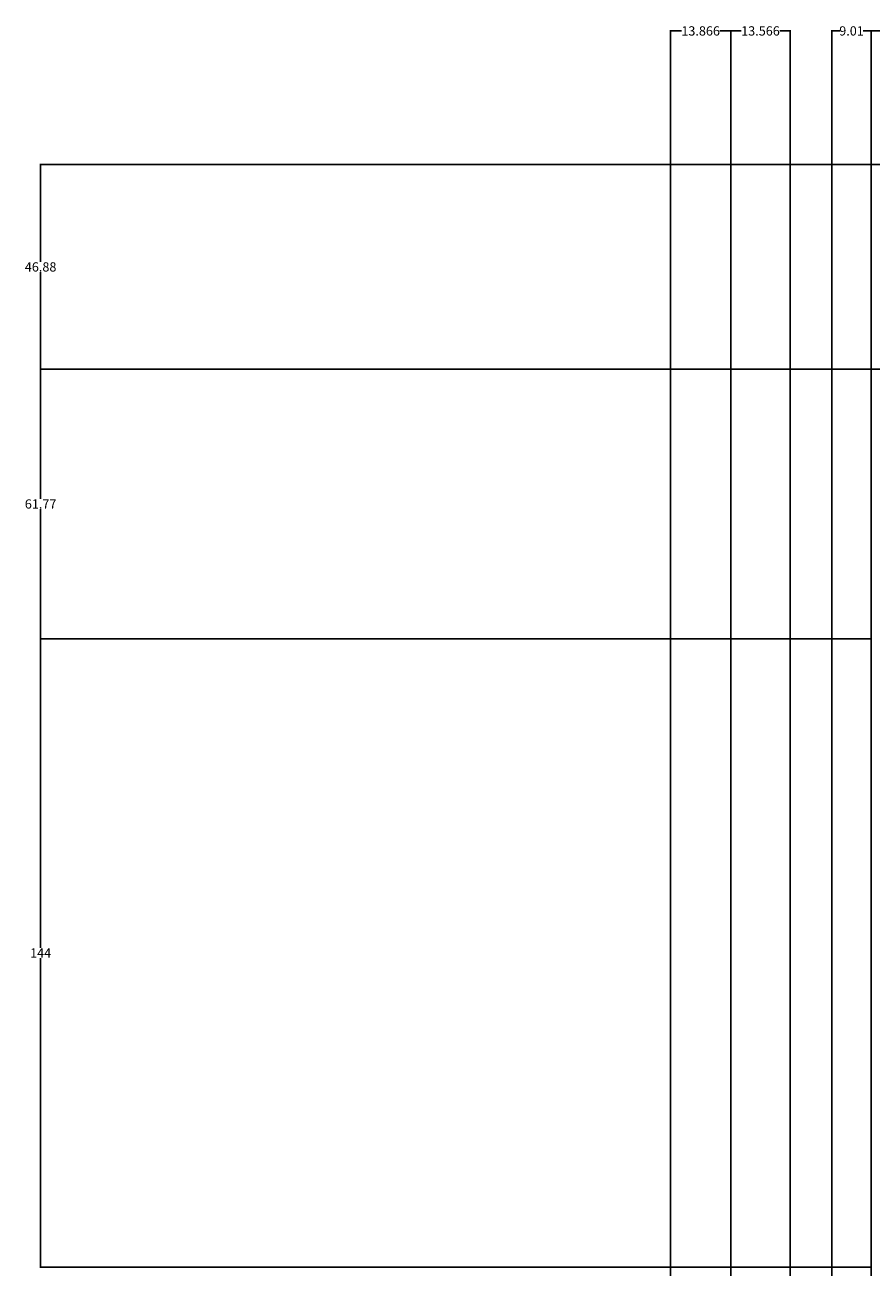
# Model space of a CAD drawing. Units: inches. Extents: x -113 to 379, y 13 to 689.
# Tile 4 of 5: x -112 to 82, y 405 to 689. Entities that reach past the tile are written whole.
import ezdxf

# ---------------------------------------------------------------- set-up
doc = ezdxf.new("R2010")
doc.units = ezdxf.units.IN
doc.header["$MEASUREMENT"] = 0
doc.layers.add('A-ANNO-DIMS', color=2, linetype='Continuous', lineweight=18)
doc.styles.get("Standard").update_dxf_attribs({"font": 'arial.ttf'})
doc.dimstyles.get("Standard").update_dxf_attribs({"dimtxt": 2.125, "dimasz": 0.18, "dimexe": 0.18, "dimexo": 0.0625, "dimgap": 0.09, "dimtad": 0, "dimtih": 1, "dimtoh": 1, "dimdec": 4, "dimzin": 0, "dimdsep": 46, "dimlunit": 4, "dimtxsty": 'Standard', "dimcen": 0.09, "dimadec": 0, "dimazin": 0, "dimtfac": 1, "dimtdec": 4, "dimtofl": 0, "dimtmove": 0, "dimatfit": 3, "dimfxl": 1, "dimtolj": 1, "dimtzin": 0, "dimarcsym": 0})

# ---------------------------------------------------------------- blocks, each defined once
blk = doc.blocks.new('*D21')
at = {"layer": 'A-ANNO-DIMS', "color": 0, "lineweight": -2, "transparency": 16777216}
for p, q in [((232.62, 657.3), (-108.66, 657.3)), ((-108.48, 657.12), (-108.48, 635.04)), ((-108.48, 610.6), (-108.48, 632.69)), ((121.43, 610.42), (-108.66, 610.42))]:
    blk.add_line(p, q, dxfattribs=at)
at = {"layer": 'A-ANNO-DIMS', "color": 0, "transparency": 16777216}
for points in [[(-108.51, 657.12), (-108.45, 657.12), (-108.48, 657.3)], [(-108.51, 610.6), (-108.45, 610.6), (-108.48, 610.42)]]:
    blk.add_solid(points, dxfattribs=at)
at = {"layer": 'Defpoints', "color": 0, "transparency": 16777216}
for p in [(-108.48, 657.3), (232.68, 657.3), (121.49, 610.42)]:
    blk.add_point(p, dxfattribs=at)
at = {"layer": 'A-ANNO-DIMS', "color": 0, "transparency": 16777216, "insert": (-108.48, 633.86), "char_height": 2.125, "attachment_point": 5}
blk.add_mtext('\\A1;46.88', dxfattribs=at)
blk = doc.blocks.new('*D23')
at = {"layer": 'A-ANNO-DIMS', "color": 0, "lineweight": -2, "transparency": 16777216}
for p, q in [((81.87, 548.71), (81.87, 688.12)), ((82.05, 687.94), (98.02, 687.94)), ((121.31, 687.94), (105.34, 687.94)), ((121.49, 610.48), (121.49, 688.12))]:
    blk.add_line(p, q, dxfattribs=at)
at = {"layer": 'A-ANNO-DIMS', "color": 0, "transparency": 16777216}
for points in [[(82.05, 687.97), (82.05, 687.91), (81.87, 687.94)], [(121.31, 687.97), (121.31, 687.91), (121.49, 687.94)]]:
    blk.add_solid(points, dxfattribs=at)
at = {"layer": 'Defpoints', "color": 0, "transparency": 16777216}
for p in [(121.49, 687.94), (121.49, 610.42), (81.87, 548.65)]:
    blk.add_point(p, dxfattribs=at)
at = {"layer": 'A-ANNO-DIMS', "color": 0, "transparency": 16777216, "insert": (101.68, 687.94), "char_height": 2.125, "attachment_point": 5}
blk.add_mtext('\\A1;39.62', dxfattribs=at)
blk = doc.blocks.new('*D28')
at = {"layer": 'A-ANNO-DIMS', "color": 0, "lineweight": -2, "transparency": 16777216}
for p, q in [((121.43, 610.42), (-108.66, 610.42)), ((-108.48, 610.24), (-108.48, 580.71)), ((-108.48, 548.83), (-108.48, 578.36)), ((81.81, 548.65), (-108.66, 548.65))]:
    blk.add_line(p, q, dxfattribs=at)
at = {"layer": 'A-ANNO-DIMS', "color": 0, "transparency": 16777216}
for points in [[(-108.51, 610.24), (-108.45, 610.24), (-108.48, 610.42)], [(-108.51, 548.83), (-108.45, 548.83), (-108.48, 548.65)]]:
    blk.add_solid(points, dxfattribs=at)
at = {"layer": 'Defpoints', "color": 0, "transparency": 16777216}
for p in [(-108.48, 610.42), (121.49, 610.42), (81.87, 548.65)]:
    blk.add_point(p, dxfattribs=at)
at = {"layer": 'A-ANNO-DIMS', "color": 0, "transparency": 16777216, "insert": (-108.48, 579.54), "char_height": 2.125, "attachment_point": 5}
blk.add_mtext('\\A1;61.77', dxfattribs=at)
blk = doc.blocks.new('*D29')
at = {"layer": 'A-ANNO-DIMS', "color": 0, "lineweight": -2, "transparency": 16777216}
for p, q in [((81.81, 548.65), (-108.66, 548.65)), ((-108.48, 548.47), (-108.48, 477.81)), ((-108.48, 404.83), (-108.48, 475.49)), ((81.81, 404.65), (-108.66, 404.65))]:
    blk.add_line(p, q, dxfattribs=at)
at = {"layer": 'A-ANNO-DIMS', "color": 0, "transparency": 16777216}
for points in [[(-108.51, 548.47), (-108.45, 548.47), (-108.48, 548.65)], [(-108.51, 404.83), (-108.45, 404.83), (-108.48, 404.65)]]:
    blk.add_solid(points, dxfattribs=at)
at = {"layer": 'Defpoints', "color": 0, "transparency": 16777216}
for p in [(-108.48, 548.65), (81.87, 548.65), (81.87, 404.65)]:
    blk.add_point(p, dxfattribs=at)
at = {"layer": 'A-ANNO-DIMS', "color": 0, "transparency": 16777216, "insert": (-108.48, 476.65), "char_height": 2.125, "attachment_point": 5}
blk.add_mtext('\\A1;144', dxfattribs=at)
blk = doc.blocks.new('*D50')
at = {"layer": 'A-ANNO-DIMS', "color": 0, "lineweight": -2, "transparency": 16777216}
for p, q in [((72.86, 171.91), (72.86, 688.12)), ((73.04, 687.94), (74.72, 687.94)), ((81.69, 687.94), (80.01, 687.94)), ((81.87, 180.47), (81.87, 688.12))]:
    blk.add_line(p, q, dxfattribs=at)
at = {"layer": 'A-ANNO-DIMS', "color": 0, "transparency": 16777216}
for points in [[(73.04, 687.97), (73.04, 687.91), (72.86, 687.94)], [(81.69, 687.97), (81.69, 687.91), (81.87, 687.94)]]:
    blk.add_solid(points, dxfattribs=at)
at = {"layer": 'Defpoints', "color": 0, "transparency": 16777216}
for p in [(81.87, 687.94), (81.87, 180.4), (72.86, 171.85)]:
    blk.add_point(p, dxfattribs=at)
at = {"layer": 'A-ANNO-DIMS', "color": 0, "transparency": 16777216, "insert": (77.37, 687.94), "char_height": 2.125, "attachment_point": 5}
blk.add_mtext('\\A1;9.01', dxfattribs=at)
blk = doc.blocks.new('*D71')
at = {"layer": 'A-ANNO-DIMS', "color": 0, "lineweight": -2, "transparency": 16777216}
for p, q in [((35.86, 169.91), (35.86, 688.12)), ((36.04, 687.94), (38.39, 687.94)), ((49.55, 687.94), (47.19, 687.94)), ((49.73, 169.91), (49.73, 688.12))]:
    blk.add_line(p, q, dxfattribs=at)
at = {"layer": 'A-ANNO-DIMS', "color": 0, "transparency": 16777216}
for points in [[(36.04, 687.97), (36.04, 687.91), (35.86, 687.94)], [(49.55, 687.97), (49.55, 687.91), (49.73, 687.94)]]:
    blk.add_solid(points, dxfattribs=at)
at = {"layer": 'Defpoints', "color": 0, "transparency": 16777216}
for p in [(49.73, 687.94), (35.86, 169.85), (49.73, 169.85)]:
    blk.add_point(p, dxfattribs=at)
at = {"layer": 'A-ANNO-DIMS', "color": 0, "transparency": 16777216, "insert": (42.79, 687.94), "char_height": 2.125, "attachment_point": 5}
blk.add_mtext('\\A1;13.866', dxfattribs=at)
blk = doc.blocks.new('*D72')
at = {"layer": 'A-ANNO-DIMS', "color": 0, "lineweight": -2, "transparency": 16777216}
for p, q in [((49.73, 169.91), (49.73, 688.12)), ((49.91, 687.94), (52.11, 687.94)), ((63.11, 687.94), (60.91, 687.94)), ((63.29, 169.91), (63.29, 688.12))]:
    blk.add_line(p, q, dxfattribs=at)
at = {"layer": 'A-ANNO-DIMS', "color": 0, "transparency": 16777216}
for points in [[(49.91, 687.97), (49.91, 687.91), (49.73, 687.94)], [(63.11, 687.97), (63.11, 687.91), (63.29, 687.94)]]:
    blk.add_solid(points, dxfattribs=at)
at = {"layer": 'Defpoints', "color": 0, "transparency": 16777216}
for p in [(63.29, 687.94), (49.73, 169.85), (63.29, 169.85)]:
    blk.add_point(p, dxfattribs=at)
at = {"layer": 'A-ANNO-DIMS', "color": 0, "transparency": 16777216, "insert": (56.51, 687.94), "char_height": 2.125, "attachment_point": 5}
blk.add_mtext('\\A1;13.566', dxfattribs=at)

msp = doc.modelspace()

# ---------------------------------------------------------------- dimensions: what is measured, and where the dimension line sits
at = {"layer": 'A-ANNO-DIMS'}
for base, p1, p2, override, picture, middle in [((49.7256, 687.9364), (35.86, 169.8462), (49.7256, 169.8462), {"dimdec": 3, "dimlfac": 1, "dimrnd": 0, "dimzin": 0, "dimdsep": 46, "dimlunit": 2}, '*D71', (42.7928, 687.9364)), ((63.2917, 687.9364), (49.7256, 169.8462), (63.2917, 169.8462), {"dimdec": 3, "dimlfac": 1, "dimrnd": 0, "dimzin": 0, "dimdsep": 46, "dimlunit": 2}, '*D72', (56.5087, 687.9364)), ((81.8721, 687.9364), (72.8619, 171.8462), (81.8721, 180.405), {"dimdec": 2, "dimlfac": 1, "dimrnd": 0, "dimzin": 0, "dimdsep": 46, "dimlunit": 2}, '*D50', (77.367, 687.9364)), ((121.4902, 687.9364), (81.8721, 548.6509), (121.4902, 610.4218), {"dimdec": 2, "dimlfac": 1, "dimrnd": 0, "dimzin": 0, "dimdsep": 46, "dimlunit": 2}, '*D23', (101.6811, 687.9364))]:
    dim = msp.add_linear_dim(base=base, p1=p1, p2=p2, dimstyle='Standard', override=override, dxfattribs=at)
    dim.commit()
    dim.dimension.update_dxf_attribs({"geometry": picture, "text_midpoint": middle})
for base, p1, p2, override, picture, middle in [((-108.4772, 657.3014), (121.4902, 610.4218), (232.6797, 657.3014), {"dimdec": 2, "dimlfac": 1, "dimrnd": 0, "dimzin": 0, "dimdsep": 46, "dimlunit": 2}, '*D21', (-108.4772, 633.8616)), ((-108.4772, 610.4218), (81.8721, 548.6509), (121.4902, 610.4218), {"dimdec": 2, "dimlfac": 1, "dimrnd": 0, "dimzin": 0, "dimdsep": 46, "dimlunit": 2}, '*D28', (-108.4772, 579.5364)), ((-108.4772, 548.6509), (81.8721, 404.6509), (81.8721, 548.6509), {"dimdec": 0, "dimlfac": 1, "dimrnd": 0, "dimzin": 0, "dimdsep": 46, "dimlunit": 2}, '*D29', (-108.4772, 476.6509))]:
    dim = msp.add_linear_dim(base=base, p1=p1, p2=p2, angle=90, dimstyle='Standard', override=override, dxfattribs=at)
    dim.commit()
    dim.dimension.update_dxf_attribs({"geometry": picture, "text_midpoint": middle})

doc.saveas('drawing.dxf')
